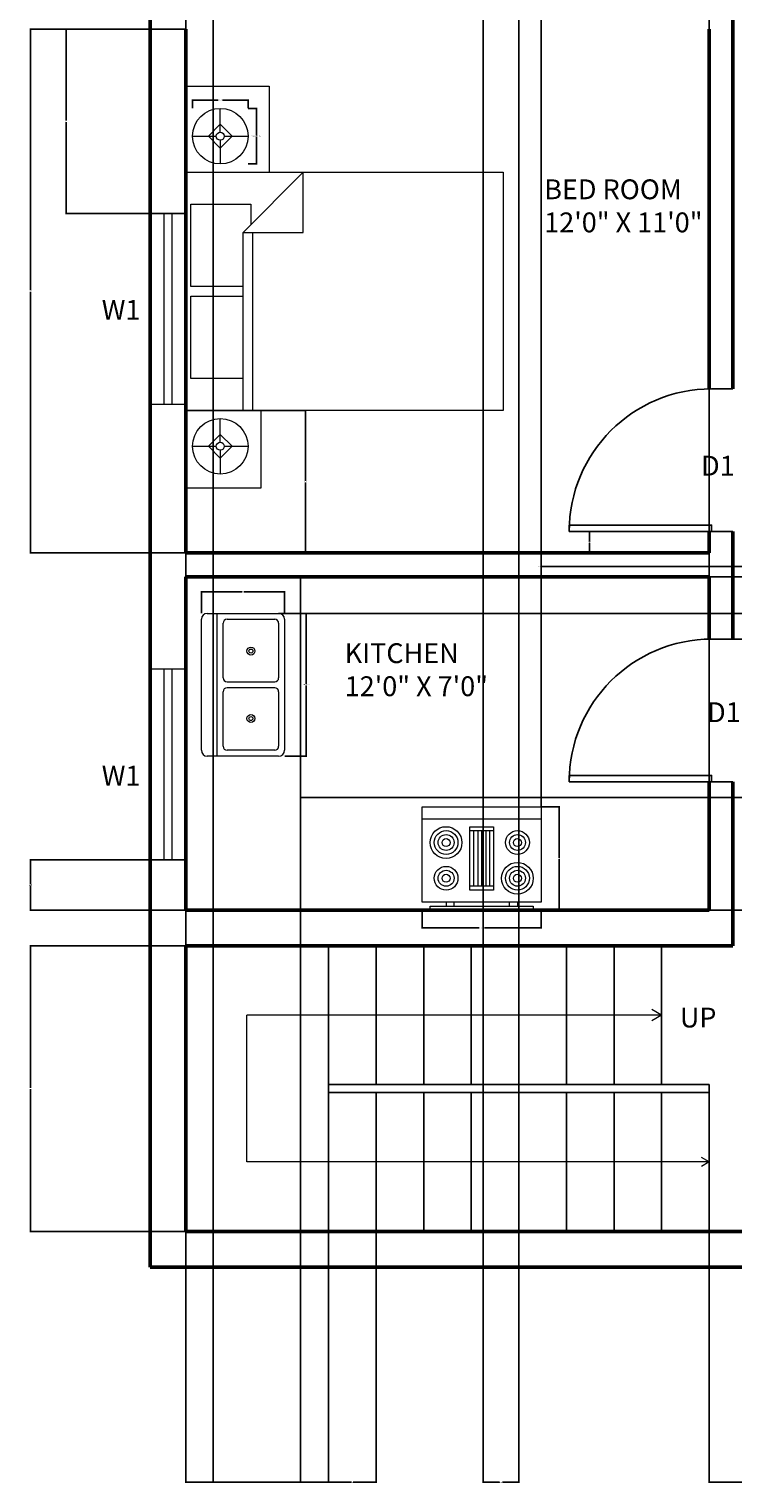
# Model space of a CAD drawing. Units: inches. Extents: x 437 to 811, y 2074 to 2699.
# Tile 1 of 4: x 437 to 615, y 2074 to 2441. Entities that reach past the tile are written whole.
import ezdxf

# ---------------------------------------------------------------- set-up
doc = ezdxf.new("R2010")
doc.units = ezdxf.units.IN
for name, color, linetype, lineweight in [('A-ANNO-DIMS', 2, 'Continuous', 18), ('A-ANNO-SYMB', 3, 'Continuous', 18), ('A-ANNO-TEXT', 7, 'Continuous', 18), ('A-AREA-IDEN', 7, 'Continuous', 25), ('A-DOOR', 4, 'Continuous', 25), ('A-EQPM', 8, 'Continuous', 18), ('A-FLOR-CASE', 9, 'Continuous', 25), ('A-FLOR-FIXT', 9, 'Continuous', 18), ('A-FLOR-STRS', 7, 'Continuous', 25), ('A-FURN', 8, 'Continuous', 18), ('A-GLAZ', 4, 'Continuous', 18), ('A-WALL', 7, 'Continuous', 50)]:
    doc.layers.add(name, color=color, linetype=linetype, lineweight=lineweight)
doc.styles.get("Standard").update_dxf_attribs({"font": 'arial.ttf'})
doc.dimstyles.get("Standard").update_dxf_attribs({"dimtxt": 0.18, "dimasz": 0.18, "dimexe": 0.18, "dimexo": 0.0625, "dimgap": 0.09, "dimtad": 0, "dimtih": 1, "dimtoh": 1, "dimdec": 4, "dimzin": 0, "dimdsep": 46, "dimtxsty": 'Standard', "dimcen": 0.09, "dimadec": 0, "dimazin": 0, "dimtfac": 1, "dimtdec": 4, "dimtofl": 0, "dimtmove": 0, "dimatfit": 3, "dimfxl": 1, "dimtolj": 1, "dimtzin": 0, "dimarcsym": 0})

# ---------------------------------------------------------------- blocks, each defined once
blk = doc.blocks.new('Range-Oven - 30 in top')
for p, q in [((0, -3), (30, -3)), ((12, -6), (18, -6)), ((13, -20), (13, -6)), ((14, -6), (14, -20)), ((15, -20), (15, -6)), ((16, -6), (16, -20)), ((17, -20), (17, -6)), ((18, -20), (12, -20)), ((6, -24), (6, -25)), ((8, -25), (8, -24)), ((22, -25), (22, -24)), ((24, -24), (24, -25))]:
    blk.add_line(p, q)
for points in [[(0, -24), (0, 0), (30, 0), (30, -24)], [(12, -21), (12, -5), (18, -5), (18, -21)], [(2, -26), (2, -25), (28, -25), (28, -26)]]:
    blk.add_lwpolyline(points, close=True)
for centre, radius in [((6, -9), 4), ((6, -9), 3), ((6, -9), 2), ((24, -9), 3), ((24, -9), 2), ((6, -9), 1), ((24, -9), 1), ((24, -18), 4), ((6, -18), 3), ((6, -18), 2), ((6, -18), 1), ((24, -18), 3), ((24, -18), 2), ((24, -18), 1)]:
    blk.add_circle(centre, radius)
blk = doc.blocks.new('Sink-double - 36 in top')
for p, q in [((-18, -4), (18, -4)), ((-0.75, -18.5), (-0.75, -6.5)), ((0.75, -6.5), (0.75, -18.5))]:
    blk.add_line(p, q)
for points in [[(-16.5, 0), (16.5, 0)], [(-18, -19.5), (-18, -1.5)], [(18, -1.5), (18, -19.5)], [(-16.5, -18.5), (-16.5, -6.5)], [(-15.5, -5.5), (-1.75, -5.5)], [(1.75, -5.5), (15.5, -5.5)], [(16.5, -6.5), (16.5, -18.5)], [(16.5, -21), (-16.5, -21)], [(-1.75, -19.5), (-15.5, -19.5)], [(15.5, -19.5), (1.75, -19.5)]]:
    blk.add_lwpolyline(points)
for centre, radius in [((-8.5, -12.5), 1), ((-8.5, -12.5), 0.5), ((8.5, -12.5), 1), ((8.5, -12.5), 0.5)]:
    blk.add_circle(centre, radius)
for centre, radius, start, end in [((-16.5, -1.5), 1.5, 90, 180), ((16.5, -1.5), 1.5, 0, 90), ((-15.5, -6.5), 1, 90, 180), ((-1.75, -6.5), 1, 0, 90), ((1.75, -6.5), 1, 90, 180), ((15.5, -6.5), 1, 0, 90), ((-16.5, -19.5), 1.5, 180, 270), ((-15.5, -18.5), 1, 180, 270), ((-1.75, -18.5), 1, 270, 0), ((1.75, -18.5), 1, 180, 270), ((15.5, -18.5), 1, 270, 0), ((16.5, -19.5), 1.5, 270, 0)]:
    blk.add_arc(centre, radius, start, end)
blk = doc.blocks.new('Bed - Queen')
for p, q in [((0, -80.00003), (0, 0)), ((0, 0), (59.99999, 0)), ((59.99999, 0), (59.99999, -80.00003)), ((7.99999, -1.2), (28.79998, -1.2)), ((7.99999, -14.4), (7.99999, -1.2)), ((28.79998, -1.2), (28.79998, -14.4)), ((31.19999, -1.2), (51.99999, -1.2)), ((31.19999, -14.4), (31.19999, -1.2)), ((51.99999, -1.2), (51.99999, -16.4)), ((0, -14.4), (44.8, -14.4)), ((59.99999, -29.6), (44.8, -14.4)), ((44.8, -14.4), (44.8, -29.6)), ((44.8, -16.8), (0, -16.8)), ((51.99999, -16.4), (46.79936, -16.4)), ((44.8, -29.6), (59.99999, -29.6)), ((59.99999, -80.00003), (0, -80.00003))]:
    blk.add_line(p, q)
blk = doc.blocks.new('Lamp - Table')
for p, q in [((0, 7), (0, 1)), ((-1, 0), (-7, 0)), ((0, 3), (-3, 0)), ((-3, 0), (0, -3)), ((3, 0), (0, 3)), ((0, -3), (3, 0)), ((1, 0), (7, 0)), ((0, -1), (0, -7))]:
    blk.add_line(p, q)
for radius in [7, 1]:
    blk.add_circle((0, 0), radius)
blk = doc.blocks.new('*U10')
for p, q in [((0, 0), (0, -6)), ((40, 0), (40, -6))]:
    blk.add_line(p, q)
blk.add_lwpolyline([(0, 0), (0, 40), (1.75, 40), (1.75, 0)], close=True)
blk.add_arc((0, 0), 40, 0, 90)
blk = doc.blocks.new('WIN-W1-48IN')
for p, q in [((0, 5.5), (48, 5.5)), ((0, 3.5), (48, 3.5))]:
    blk.add_line(p, q)
blk.add_lwpolyline([(0, 0), (48, 0), (48, 9), (0, 9)], close=True)
blk = doc.blocks.new('NIGHTSTAND-SMALL')
for p, q in [((0, 19.48), (0, 0)), ((19, 0), (19, 19.48)), ((0, 0), (19, 0))]:
    blk.add_line(p, q)
blk = doc.blocks.new('NIGHTSTAND-LARGE')
for p, q in [((0, 0), (0, 21.74)), ((0, 21.74), (21.02, 21.74)), ((21.02, 21.74), (21.02, 0))]:
    blk.add_line(p, q)
blk = doc.blocks.new('*D16')
at = {"layer": 'A-ANNO-DIMS', "color": 0, "lineweight": -2, "transparency": 16777216}
for p, q in [((492.74, 2420.81), (494.96, 2420.81)), ((494.78, 2420.63), (494.78, 2413.99)), ((494.78, 2406.99), (494.78, 2413.62)), ((492.74, 2406.81), (494.96, 2406.81))]:
    blk.add_line(p, q, dxfattribs=at)
at = {"layer": 'A-ANNO-DIMS', "color": 0, "transparency": 16777216}
for points in [[(494.75, 2420.63), (494.81, 2420.63), (494.78, 2420.81)], [(494.75, 2406.99), (494.81, 2406.99), (494.78, 2406.81)]]:
    blk.add_solid(points, dxfattribs=at)
at = {"layer": 'Defpoints', "color": 0, "transparency": 16777216}
for p in [(492.68, 2420.81), (494.78, 2420.81), (492.68, 2406.81)]:
    blk.add_point(p, dxfattribs=at)
at = {"layer": 'A-ANNO-DIMS', "color": 0, "transparency": 16777216, "insert": (494.78, 2413.81), "char_height": 0.18, "attachment_point": 5}
blk.add_mtext('\\A1;TABLE LAMP 14 TYP.', dxfattribs=at)
blk = doc.blocks.new('*D17')
at = {"layer": 'A-ANNO-DIMS', "color": 0, "lineweight": -2, "transparency": 16777216}
for p, q in [((478.68, 2420.87), (478.68, 2423.09)), ((478.86, 2422.91), (485.16, 2422.91)), ((492.5, 2422.91), (486.2, 2422.91)), ((492.68, 2420.87), (492.68, 2423.09))]:
    blk.add_line(p, q, dxfattribs=at)
at = {"layer": 'A-ANNO-DIMS', "color": 0, "transparency": 16777216}
for points in [[(478.86, 2422.94), (478.86, 2422.88), (478.68, 2422.91)], [(492.5, 2422.94), (492.5, 2422.88), (492.68, 2422.91)]]:
    blk.add_solid(points, dxfattribs=at)
at = {"layer": 'Defpoints', "color": 0, "transparency": 16777216}
for p in [(478.68, 2422.91), (478.68, 2420.81), (492.68, 2420.81)]:
    blk.add_point(p, dxfattribs=at)
at = {"layer": 'A-ANNO-DIMS', "color": 0, "transparency": 16777216, "insert": (485.68, 2422.91), "char_height": 0.18, "attachment_point": 5}
blk.add_mtext('\\A1;14 TYP.', dxfattribs=at)
blk = doc.blocks.new('*D38')
at = {"layer": 'A-ANNO-DIMS', "color": 0, "lineweight": -2, "transparency": 16777216}
for p, q in [((536.64, 2218.74), (536.64, 2214.12)), ((566.64, 2218.74), (566.64, 2214.12)), ((536.82, 2214.3), (550.94, 2214.3)), ((566.46, 2214.3), (552.33, 2214.3))]:
    blk.add_line(p, q, dxfattribs=at)
at = {"layer": 'A-ANNO-DIMS', "color": 0, "transparency": 16777216}
for points in [[(536.82, 2214.33), (536.82, 2214.27), (536.64, 2214.3)], [(566.46, 2214.33), (566.46, 2214.27), (566.64, 2214.3)]]:
    blk.add_solid(points, dxfattribs=at)
at = {"layer": 'Defpoints', "color": 0, "transparency": 16777216}
for p in [(536.64, 2218.8), (566.64, 2218.8), (566.64, 2214.3)]:
    blk.add_point(p, dxfattribs=at)
at = {"layer": 'A-ANNO-DIMS', "color": 0, "transparency": 16777216, "insert": (551.64, 2214.3), "char_height": 0.18, "attachment_point": 5}
blk.add_mtext('\\A1;RANGE 30', dxfattribs=at)
blk = doc.blocks.new('*D39')
at = {"layer": 'A-ANNO-DIMS', "color": 0, "lineweight": -2, "transparency": 16777216}
for p, q in [((566.7, 2244.8), (571.32, 2244.8)), ((571.14, 2244.62), (571.14, 2231.98)), ((571.14, 2218.98), (571.14, 2231.62)), ((566.7, 2218.8), (571.32, 2218.8))]:
    blk.add_line(p, q, dxfattribs=at)
at = {"layer": 'A-ANNO-DIMS', "color": 0, "transparency": 16777216}
for points in [[(571.11, 2244.62), (571.17, 2244.62), (571.14, 2244.8)], [(571.11, 2218.98), (571.17, 2218.98), (571.14, 2218.8)]]:
    blk.add_solid(points, dxfattribs=at)
at = {"layer": 'Defpoints', "color": 0, "transparency": 16777216}
for p in [(566.64, 2244.8), (571.14, 2244.8), (566.64, 2218.8)]:
    blk.add_point(p, dxfattribs=at)
at = {"layer": 'A-ANNO-DIMS', "color": 0, "transparency": 16777216, "insert": (571.14, 2231.8), "char_height": 0.18, "attachment_point": 5}
blk.add_mtext('\\A1;26', dxfattribs=at)
blk = doc.blocks.new('*D40')
at = {"layer": 'A-ANNO-DIMS', "color": 0, "lineweight": -2, "transparency": 16777216}
for p, q in [((501.96, 2293.56), (507.48, 2293.56)), ((507.3, 2293.38), (507.3, 2275.74)), ((507.3, 2257.74), (507.3, 2275.37)), ((501.96, 2257.56), (507.48, 2257.56))]:
    blk.add_line(p, q, dxfattribs=at)
at = {"layer": 'A-ANNO-DIMS', "color": 0, "transparency": 16777216}
for points in [[(507.27, 2293.38), (507.33, 2293.38), (507.3, 2293.56)], [(507.27, 2257.74), (507.33, 2257.74), (507.3, 2257.56)]]:
    blk.add_solid(points, dxfattribs=at)
at = {"layer": 'Defpoints', "color": 0, "transparency": 16777216}
for p in [(501.9, 2293.56), (507.3, 2293.56), (501.9, 2257.56)]:
    blk.add_point(p, dxfattribs=at)
at = {"layer": 'A-ANNO-DIMS', "color": 0, "transparency": 16777216, "insert": (507.3, 2275.56), "char_height": 0.18, "attachment_point": 5}
blk.add_mtext('\\A1;DOUBLE SINK 36', dxfattribs=at)
blk = doc.blocks.new('*D41')
at = {"layer": 'A-ANNO-DIMS', "color": 0, "lineweight": -2, "transparency": 16777216}
for p, q in [((480.9, 2293.62), (480.9, 2299.14)), ((481.08, 2298.96), (491.2, 2298.96)), ((501.72, 2298.96), (491.6, 2298.96)), ((501.9, 2293.62), (501.9, 2299.14))]:
    blk.add_line(p, q, dxfattribs=at)
at = {"layer": 'A-ANNO-DIMS', "color": 0, "transparency": 16777216}
for points in [[(481.08, 2298.99), (481.08, 2298.93), (480.9, 2298.96)], [(501.72, 2298.99), (501.72, 2298.93), (501.9, 2298.96)]]:
    blk.add_solid(points, dxfattribs=at)
at = {"layer": 'Defpoints', "color": 0, "transparency": 16777216}
for p in [(480.9, 2298.96), (480.9, 2293.56), (501.9, 2293.56)]:
    blk.add_point(p, dxfattribs=at)
at = {"layer": 'A-ANNO-DIMS', "color": 0, "transparency": 16777216, "insert": (491.4, 2298.96), "char_height": 0.18, "attachment_point": 5}
blk.add_mtext('\\A1;21', dxfattribs=at)
blk = doc.blocks.new('*D44')
at = {"layer": 'A-ANNO-DIMS', "color": 0, "lineweight": -2, "transparency": 16777216}
for p, q in [((609, 2137.74), (609, 2074.42)), ((645.69, 2104.74), (645.69, 2074.42)), ((609.18, 2074.6), (626.95, 2074.6)), ((645.51, 2074.6), (627.74, 2074.6))]:
    blk.add_line(p, q, dxfattribs=at)
at = {"layer": 'A-ANNO-DIMS', "color": 0, "transparency": 16777216}
for points in [[(609.18, 2074.63), (609.18, 2074.57), (609, 2074.6)], [(645.51, 2074.63), (645.51, 2074.57), (645.69, 2074.6)]]:
    blk.add_solid(points, dxfattribs=at)
at = {"layer": 'Defpoints', "color": 0, "transparency": 16777216}
for p in [(609, 2137.8), (645.69, 2104.8), (645.69, 2074.6)]:
    blk.add_point(p, dxfattribs=at)
at = {"layer": 'A-ANNO-DIMS', "color": 0, "transparency": 16777216, "insert": (627.35, 2074.6), "char_height": 0.18, "attachment_point": 5}
blk.add_mtext('\\A1;36.69', dxfattribs=at)
blk = doc.blocks.new('*D51')
at = {"layer": 'A-ANNO-DIMS', "color": 0, "lineweight": -2, "transparency": 16777216}
for p, q in [((476.94, 2231.48), (437.62, 2231.48)), ((437.8, 2231.3), (437.8, 2225.32)), ((437.8, 2218.98), (437.8, 2224.96)), ((476.94, 2218.8), (437.62, 2218.8))]:
    blk.add_line(p, q, dxfattribs=at)
at = {"layer": 'A-ANNO-DIMS', "color": 0, "transparency": 16777216}
for points in [[(437.77, 2231.3), (437.83, 2231.3), (437.8, 2231.48)], [(437.77, 2218.98), (437.83, 2218.98), (437.8, 2218.8)]]:
    blk.add_solid(points, dxfattribs=at)
at = {"layer": 'Defpoints', "color": 0, "transparency": 16777216}
for p in [(437.8, 2231.48), (477, 2231.48), (477, 2218.8)]:
    blk.add_point(p, dxfattribs=at)
at = {"layer": 'A-ANNO-DIMS', "color": 0, "transparency": 16777216, "insert": (437.8, 2225.14), "char_height": 0.18, "attachment_point": 5}
blk.add_mtext('\\A1;12.684', dxfattribs=at)
blk = doc.blocks.new('*D52')
at = {"layer": 'A-ANNO-DIMS', "color": 0, "lineweight": -2, "transparency": 16777216}
for p, q in [((476.94, 2440.8), (446.62, 2440.8)), ((446.8, 2440.62), (446.8, 2417.73)), ((446.8, 2394.48), (446.8, 2417.37)), ((476.94, 2394.3), (446.62, 2394.3))]:
    blk.add_line(p, q, dxfattribs=at)
at = {"layer": 'A-ANNO-DIMS', "color": 0, "transparency": 16777216}
for points in [[(446.77, 2440.62), (446.83, 2440.62), (446.8, 2440.8)], [(446.77, 2394.48), (446.83, 2394.48), (446.8, 2394.3)]]:
    blk.add_solid(points, dxfattribs=at)
at = {"layer": 'Defpoints', "color": 0, "transparency": 16777216}
for p in [(446.8, 2440.8), (477, 2440.8), (477, 2394.3)]:
    blk.add_point(p, dxfattribs=at)
at = {"layer": 'A-ANNO-DIMS', "color": 0, "transparency": 16777216, "insert": (446.8, 2417.55), "char_height": 0.18, "attachment_point": 5}
blk.add_mtext('\\A1;46.5', dxfattribs=at)
blk = doc.blocks.new('*D53')
at = {"layer": 'A-ANNO-DIMS', "color": 0, "lineweight": -2, "transparency": 16777216}
for p, q in [((476.94, 2440.8), (437.62, 2440.8)), ((437.8, 2440.62), (437.8, 2374.98)), ((437.8, 2308.98), (437.8, 2374.62)), ((476.94, 2308.8), (437.62, 2308.8))]:
    blk.add_line(p, q, dxfattribs=at)
at = {"layer": 'A-ANNO-DIMS', "color": 0, "transparency": 16777216}
for points in [[(437.77, 2440.62), (437.83, 2440.62), (437.8, 2440.8)], [(437.77, 2308.98), (437.83, 2308.98), (437.8, 2308.8)]]:
    blk.add_solid(points, dxfattribs=at)
at = {"layer": 'Defpoints', "color": 0, "transparency": 16777216}
for p in [(437.8, 2440.8), (477, 2440.8), (477, 2308.8)]:
    blk.add_point(p, dxfattribs=at)
at = {"layer": 'A-ANNO-DIMS', "color": 0, "transparency": 16777216, "insert": (437.8, 2374.8), "char_height": 0.18, "attachment_point": 5}
blk.add_mtext('\\A1;132', dxfattribs=at)
blk = doc.blocks.new('*D61')
at = {"layer": 'A-ANNO-DIMS', "color": 0, "lineweight": -2, "transparency": 16777216}
for p, q in [((476.94, 2209.8), (437.62, 2209.8)), ((437.8, 2209.62), (437.8, 2173.98)), ((437.8, 2137.98), (437.8, 2173.62)), ((476.94, 2137.8), (437.62, 2137.8))]:
    blk.add_line(p, q, dxfattribs=at)
at = {"layer": 'A-ANNO-DIMS', "color": 0, "transparency": 16777216}
for points in [[(437.77, 2209.62), (437.83, 2209.62), (437.8, 2209.8)], [(437.77, 2137.98), (437.83, 2137.98), (437.8, 2137.8)]]:
    blk.add_solid(points, dxfattribs=at)
at = {"layer": 'Defpoints', "color": 0, "transparency": 16777216}
for p in [(437.8, 2209.8), (477, 2209.8), (477, 2137.8)]:
    blk.add_point(p, dxfattribs=at)
at = {"layer": 'A-ANNO-DIMS', "color": 0, "transparency": 16777216, "insert": (437.8, 2173.8), "char_height": 0.18, "attachment_point": 5}
blk.add_mtext('\\A1;72', dxfattribs=at)
blk = doc.blocks.new('*D62')
at = {"layer": 'A-ANNO-DIMS', "color": 0, "lineweight": -2, "transparency": 16777216}
for p, q in [((477, 2137.74), (477, 2074.42)), ((513, 2137.74), (513, 2074.42)), ((477.18, 2074.6), (494.79, 2074.6)), ((512.82, 2074.6), (495.22, 2074.6))]:
    blk.add_line(p, q, dxfattribs=at)
at = {"layer": 'A-ANNO-DIMS', "color": 0, "transparency": 16777216}
for points in [[(477.18, 2074.63), (477.18, 2074.57), (477, 2074.6)], [(512.82, 2074.63), (512.82, 2074.57), (513, 2074.6)]]:
    blk.add_solid(points, dxfattribs=at)
at = {"layer": 'Defpoints', "color": 0, "transparency": 16777216}
for p in [(477, 2137.8), (513, 2137.8), (513, 2074.6)]:
    blk.add_point(p, dxfattribs=at)
at = {"layer": 'A-ANNO-DIMS', "color": 0, "transparency": 16777216, "insert": (495, 2074.6), "char_height": 0.18, "attachment_point": 5}
blk.add_mtext('\\A1;36', dxfattribs=at)
blk = doc.blocks.new('*D63')
at = {"layer": 'A-ANNO-DIMS', "color": 0, "lineweight": -2, "transparency": 16777216}
for p, q in [((513, 2137.74), (513, 2074.42)), ((525, 2137.74), (525, 2074.42)), ((513.18, 2074.6), (518.8, 2074.6)), ((524.82, 2074.6), (519.21, 2074.6))]:
    blk.add_line(p, q, dxfattribs=at)
at = {"layer": 'A-ANNO-DIMS', "color": 0, "transparency": 16777216}
for points in [[(513.18, 2074.63), (513.18, 2074.57), (513, 2074.6)], [(524.82, 2074.63), (524.82, 2074.57), (525, 2074.6)]]:
    blk.add_solid(points, dxfattribs=at)
at = {"layer": 'Defpoints', "color": 0, "transparency": 16777216}
for p in [(513, 2137.8), (525, 2137.8), (525, 2074.6)]:
    blk.add_point(p, dxfattribs=at)
at = {"layer": 'A-ANNO-DIMS', "color": 0, "transparency": 16777216, "insert": (519, 2074.6), "char_height": 0.18, "attachment_point": 5}
blk.add_mtext('\\A1;12', dxfattribs=at)
blk = doc.blocks.new('*D65')
at = {"layer": 'A-ANNO-DIMS', "color": 0, "lineweight": -2, "transparency": 16777216}
for p, q in [((609.07, 2302.8), (810.38, 2302.8)), ((810.2, 2302.62), (810.2, 2295.11)), ((810.2, 2287.23), (810.2, 2294.74)), ((609.07, 2287.05), (810.38, 2287.05))]:
    blk.add_line(p, q, dxfattribs=at)
at = {"layer": 'A-ANNO-DIMS', "color": 0, "transparency": 16777216}
for points in [[(810.17, 2302.62), (810.23, 2302.62), (810.2, 2302.8)], [(810.17, 2287.23), (810.23, 2287.23), (810.2, 2287.05)]]:
    blk.add_solid(points, dxfattribs=at)
at = {"layer": 'Defpoints', "color": 0, "transparency": 16777216}
for p in [(609, 2302.8), (810.2, 2302.8), (609, 2287.05)]:
    blk.add_point(p, dxfattribs=at)
at = {"layer": 'A-ANNO-DIMS', "color": 0, "transparency": 16777216, "insert": (810.2, 2294.93), "char_height": 0.18, "attachment_point": 5}
blk.add_mtext('\\A1;15.747', dxfattribs=at)
blk = doc.blocks.new('*D66')
at = {"layer": 'A-ANNO-DIMS', "color": 0, "lineweight": -2, "transparency": 16777216}
for p, q in [((477, 2302.86), (477, 2690.18)), ((477.18, 2690), (542.73, 2690)), ((608.82, 2690), (543.28, 2690)), ((609, 2302.86), (609, 2690.18))]:
    blk.add_line(p, q, dxfattribs=at)
at = {"layer": 'A-ANNO-DIMS', "color": 0, "transparency": 16777216}
for points in [[(477.18, 2690.03), (477.18, 2689.97), (477, 2690)], [(608.82, 2690.03), (608.82, 2689.97), (609, 2690)]]:
    blk.add_solid(points, dxfattribs=at)
at = {"layer": 'Defpoints', "color": 0, "transparency": 16777216}
for p in [(609, 2690), (477, 2302.8), (609, 2302.8)]:
    blk.add_point(p, dxfattribs=at)
at = {"layer": 'A-ANNO-DIMS', "color": 0, "transparency": 16777216, "insert": (543, 2690), "char_height": 0.18, "attachment_point": 5}
blk.add_mtext('\\A1;132', dxfattribs=at)
blk = doc.blocks.new('*D67')
at = {"layer": 'A-ANNO-DIMS', "color": 0, "lineweight": -2, "transparency": 16777216}
for p, q in [((505.92, 2247.12), (505.92, 2074.42)), ((477, 2218.74), (477, 2074.42)), ((477.18, 2074.6), (491, 2074.6)), ((505.74, 2074.6), (491.93, 2074.6))]:
    blk.add_line(p, q, dxfattribs=at)
at = {"layer": 'A-ANNO-DIMS', "color": 0, "transparency": 16777216}
for points in [[(477.18, 2074.63), (477.18, 2074.57), (477, 2074.6)], [(505.74, 2074.63), (505.74, 2074.57), (505.92, 2074.6)]]:
    blk.add_solid(points, dxfattribs=at)
at = {"layer": 'Defpoints', "color": 0, "transparency": 16777216}
for p in [(505.92, 2247.18), (477, 2218.8), (505.92, 2074.6)]:
    blk.add_point(p, dxfattribs=at)
at = {"layer": 'A-ANNO-DIMS', "color": 0, "transparency": 16777216, "insert": (491.46, 2074.6), "char_height": 0.18, "attachment_point": 5}
blk.add_mtext('\\A1;28.916', dxfattribs=at)
blk = doc.blocks.new('*D68')
at = {"layer": 'A-ANNO-DIMS', "color": 0, "lineweight": -2, "transparency": 16777216}
for p, q in [((609.07, 2247.18), (810.38, 2247.18)), ((810.2, 2247), (810.2, 2233.17)), ((810.2, 2218.98), (810.2, 2232.81)), ((609.07, 2218.8), (810.38, 2218.8))]:
    blk.add_line(p, q, dxfattribs=at)
at = {"layer": 'A-ANNO-DIMS', "color": 0, "transparency": 16777216}
for points in [[(810.17, 2247), (810.23, 2247), (810.2, 2247.18)], [(810.17, 2218.98), (810.23, 2218.98), (810.2, 2218.8)]]:
    blk.add_solid(points, dxfattribs=at)
at = {"layer": 'Defpoints', "color": 0, "transparency": 16777216}
for p in [(609, 2247.18), (810.2, 2247.18), (609, 2218.8)]:
    blk.add_point(p, dxfattribs=at)
at = {"layer": 'A-ANNO-DIMS', "color": 0, "transparency": 16777216, "insert": (810.2, 2232.99), "char_height": 0.18, "attachment_point": 5}
blk.add_mtext('\\A1;28.384', dxfattribs=at)
blk = doc.blocks.new('*D69')
at = {"layer": 'A-ANNO-DIMS', "color": 0, "lineweight": -2, "transparency": 16777216}
for p, q in [((566.64, 2244.86), (566.64, 2690.18)), ((566.82, 2690), (587.42, 2690)), ((608.82, 2690), (588.22, 2690)), ((609, 2247.25), (609, 2690.18))]:
    blk.add_line(p, q, dxfattribs=at)
at = {"layer": 'A-ANNO-DIMS', "color": 0, "transparency": 16777216}
for points in [[(566.82, 2690.03), (566.82, 2689.97), (566.64, 2690)], [(608.82, 2690.03), (608.82, 2689.97), (609, 2690)]]:
    blk.add_solid(points, dxfattribs=at)
at = {"layer": 'Defpoints', "color": 0, "transparency": 16777216}
for p in [(609, 2690), (609, 2247.18), (566.64, 2244.8)]:
    blk.add_point(p, dxfattribs=at)
at = {"layer": 'A-ANNO-DIMS', "color": 0, "transparency": 16777216, "insert": (587.82, 2690), "char_height": 0.18, "attachment_point": 5}
blk.add_mtext('\\A1;42.37', dxfattribs=at)
blk = doc.blocks.new('*D70')
at = {"layer": 'A-ANNO-DIMS', "color": 0, "lineweight": -2, "transparency": 16777216}
for p, q in [((505.98, 2302.8), (810.38, 2302.8)), ((810.2, 2302.62), (810.2, 2298.36)), ((810.2, 2293.74), (810.2, 2298)), ((500.46, 2293.56), (810.38, 2293.56))]:
    blk.add_line(p, q, dxfattribs=at)
at = {"layer": 'A-ANNO-DIMS', "color": 0, "transparency": 16777216}
for points in [[(810.17, 2302.62), (810.23, 2302.62), (810.2, 2302.8)], [(810.17, 2293.74), (810.23, 2293.74), (810.2, 2293.56)]]:
    blk.add_solid(points, dxfattribs=at)
at = {"layer": 'Defpoints', "color": 0, "transparency": 16777216}
for p in [(505.92, 2302.8), (810.2, 2302.8), (500.4, 2293.56)]:
    blk.add_point(p, dxfattribs=at)
at = {"layer": 'A-ANNO-DIMS', "color": 0, "transparency": 16777216, "insert": (810.2, 2298.18), "char_height": 0.18, "attachment_point": 5}
blk.add_mtext('\\A1;9.244', dxfattribs=at)
blk = doc.blocks.new('*D71')
at = {"layer": 'A-ANNO-DIMS', "color": 0, "lineweight": -2, "transparency": 16777216}
for p, q in [((477, 2446.74), (477, 2074.42)), ((483.87, 2446.74), (483.87, 2074.42)), ((477.18, 2074.6), (480.04, 2074.6)), ((483.69, 2074.6), (480.83, 2074.6))]:
    blk.add_line(p, q, dxfattribs=at)
at = {"layer": 'A-ANNO-DIMS', "color": 0, "transparency": 16777216}
for points in [[(477.18, 2074.63), (477.18, 2074.57), (477, 2074.6)], [(483.69, 2074.63), (483.69, 2074.57), (483.87, 2074.6)]]:
    blk.add_solid(points, dxfattribs=at)
at = {"layer": 'Defpoints', "color": 0, "transparency": 16777216}
for p in [(477, 2446.8), (483.87, 2446.8), (483.87, 2074.6)]:
    blk.add_point(p, dxfattribs=at)
at = {"layer": 'A-ANNO-DIMS', "color": 0, "transparency": 16777216, "insert": (480.44, 2074.6), "char_height": 0.18, "attachment_point": 5}
blk.add_mtext('\\A1;6.864', dxfattribs=at)
blk = doc.blocks.new('*D73')
at = {"layer": 'A-ANNO-DIMS', "color": 0, "lineweight": -2, "transparency": 16777216}
for p, q in [((551.96, 2446.74), (551.96, 2074.42)), ((561, 2446.74), (561, 2074.42)), ((552.14, 2074.6), (556.09, 2074.6)), ((560.82, 2074.6), (556.88, 2074.6))]:
    blk.add_line(p, q, dxfattribs=at)
at = {"layer": 'A-ANNO-DIMS', "color": 0, "transparency": 16777216}
for points in [[(552.14, 2074.63), (552.14, 2074.57), (551.96, 2074.6)], [(560.82, 2074.63), (560.82, 2074.57), (561, 2074.6)]]:
    blk.add_solid(points, dxfattribs=at)
at = {"layer": 'Defpoints', "color": 0, "transparency": 16777216}
for p in [(551.96, 2446.8), (561, 2446.8), (561, 2074.6)]:
    blk.add_point(p, dxfattribs=at)
at = {"layer": 'A-ANNO-DIMS', "color": 0, "transparency": 16777216, "insert": (556.48, 2074.6), "char_height": 0.18, "attachment_point": 5}
blk.add_mtext('\\A1;9.045', dxfattribs=at)
blk = doc.blocks.new('*D74')
at = {"layer": 'A-ANNO-DIMS', "color": 0, "lineweight": -2, "transparency": 16777216}
for p, q in [((608.94, 2314.22), (578.62, 2314.22)), ((578.8, 2314.04), (578.8, 2311.69)), ((608.94, 2308.8), (578.62, 2308.8)), ((578.8, 2308.98), (578.8, 2311.33))]:
    blk.add_line(p, q, dxfattribs=at)
at = {"layer": 'A-ANNO-DIMS', "color": 0, "transparency": 16777216}
for points in [[(578.77, 2314.04), (578.83, 2314.04), (578.8, 2314.22)], [(578.77, 2308.98), (578.83, 2308.98), (578.8, 2308.8)]]:
    blk.add_solid(points, dxfattribs=at)
at = {"layer": 'Defpoints', "color": 0, "transparency": 16777216}
for p in [(578.8, 2314.22), (609, 2314.22), (609, 2308.8)]:
    blk.add_point(p, dxfattribs=at)
at = {"layer": 'A-ANNO-DIMS', "color": 0, "transparency": 16777216, "insert": (578.8, 2311.51), "char_height": 0.18, "attachment_point": 5}
blk.add_mtext('\\A1;5.416', dxfattribs=at)
blk = doc.blocks.new('*D81')
at = {"layer": 'A-ANNO-DIMS', "color": 0, "lineweight": -2, "transparency": 16777216}
for p, q in [((477.07, 2344.71), (507.38, 2344.71)), ((507.2, 2344.53), (507.2, 2326.93)), ((507.2, 2308.98), (507.2, 2326.57)), ((477.07, 2308.8), (507.38, 2308.8))]:
    blk.add_line(p, q, dxfattribs=at)
at = {"layer": 'A-ANNO-DIMS', "color": 0, "transparency": 16777216}
for points in [[(507.17, 2344.53), (507.23, 2344.53), (507.2, 2344.71)], [(507.17, 2308.98), (507.23, 2308.98), (507.2, 2308.8)]]:
    blk.add_solid(points, dxfattribs=at)
at = {"layer": 'Defpoints', "color": 0, "transparency": 16777216}
for p in [(477, 2344.71), (477, 2308.8), (507.2, 2308.8)]:
    blk.add_point(p, dxfattribs=at)
at = {"layer": 'A-ANNO-DIMS', "color": 0, "transparency": 16777216, "insert": (507.2, 2326.75), "char_height": 0.18, "attachment_point": 5}
blk.add_mtext('\\A1;35.906', dxfattribs=at)
blk = doc.blocks.new('*D88')
at = {"layer": 'A-ANNO-DIMS', "color": 0, "lineweight": -2, "transparency": 16777216}
for p, q in [((568.95, 2305.38), (641.01, 2305.38)), ((762.3, 2305.38), (762.48, 2305.38)), ((762.39, 2305.29), (762.39, 2305.47))]:
    blk.add_line(p, q, dxfattribs=at)
at = {"layer": 'A-ANNO-DIMS', "color": 0, "transparency": 16777216}
blk.add_solid([(641.01, 2305.41), (641.01, 2305.35), (641.19, 2305.38)], dxfattribs=at)
at = {"layer": 'Defpoints', "color": 0, "transparency": 16777216}
for p in [(641.19, 2305.38), (762.39, 2305.38)]:
    blk.add_point(p, dxfattribs=at)
at = {"layer": 'A-ANNO-DIMS', "color": 0, "transparency": 16777216, "insert": (568.47, 2305.38), "char_height": 0.18, "attachment_point": 5}
blk.add_mtext('\\A1;R121.2', dxfattribs=at)
blk = doc.blocks.new('*D89')
at = {"layer": 'A-ANNO-DIMS', "color": 0, "lineweight": -2, "transparency": 16777216}
for p, q in [((566.64, 2305.38), (635.01, 2305.38)), ((749.35, 2305.38), (749.53, 2305.38)), ((749.44, 2305.29), (749.44, 2305.47))]:
    blk.add_line(p, q, dxfattribs=at)
at = {"layer": 'A-ANNO-DIMS', "color": 0, "transparency": 16777216}
blk.add_solid([(635.01, 2305.41), (635.01, 2305.35), (635.19, 2305.38)], dxfattribs=at)
at = {"layer": 'Defpoints', "color": 0, "transparency": 16777216}
for p in [(635.19, 2305.38), (749.44, 2305.38)]:
    blk.add_point(p, dxfattribs=at)
at = {"layer": 'A-ANNO-DIMS', "color": 0, "transparency": 16777216, "insert": (566.09, 2305.38), "char_height": 0.18, "attachment_point": 5}
blk.add_mtext('\\A1;R114.25', dxfattribs=at)

msp = doc.modelspace()

# ---------------------------------------------------------------- linework, layer by layer
at = {"layer": 'A-ANNO-SYMB'}
for p, q in [((597.0049, 2192.2995), (492.3677, 2192.2995)), ((492.3677, 2155.2995), (492.3677, 2192.2995)), ((597.0049, 2192.2995), (594.5087, 2193.7406)), ((597.0049, 2192.2995), (594.5087, 2190.8583)), ((609.0049, 2155.2995), (492.3677, 2155.2995)), ((609.0049, 2155.2995), (607.0775, 2156.4122)), ((609.0049, 2155.2995), (607.0775, 2154.1867))]:
    msp.add_line(p, q, dxfattribs=at)
at = {"layer": 'A-FLOR-CASE'}
for p, q in [((505.9211, 2302.7995), (505.9211, 2247.1838)), ((505.9211, 2247.1838), (609.0049, 2247.1838))]:
    msp.add_line(p, q, dxfattribs=at)
at = {"layer": 'A-FLOR-STRS'}
for p, q in [((477.0049, 2209.7995), (477.0049, 2137.7995)), ((513.0049, 2209.7995), (513.0049, 2137.7995)), ((525.0049, 2209.7995), (525.0049, 2174.7995)), ((537.0049, 2209.7995), (537.0049, 2174.7995)), ((549.0049, 2209.7995), (549.0049, 2174.7995)), ((561.0049, 2209.7995), (561.0049, 2174.7995)), ((573.0049, 2209.7995), (573.0049, 2174.7995)), ((585.0049, 2209.7995), (585.0049, 2174.7995)), ((597.0049, 2209.7995), (597.0049, 2174.7995)), ((609.0049, 2174.7995), (513.0049, 2174.7995)), ((609.0049, 2172.7995), (513.0049, 2172.7995)), ((525.0049, 2172.7995), (525.0049, 2137.7995)), ((537.0049, 2172.7995), (537.0049, 2137.7995)), ((549.0049, 2172.7995), (549.0049, 2137.7995)), ((561.0049, 2172.7995), (561.0049, 2137.7995)), ((573.0049, 2172.7995), (573.0049, 2137.7995)), ((585.0049, 2172.7995), (585.0049, 2137.7995)), ((597.0049, 2172.7995), (597.0049, 2137.7995)), ((609.0049, 2174.7995), (609.0049, 2172.7995)), ((609.0049, 2172.7995), (609.0049, 2137.7995))]:
    msp.add_line(p, q, dxfattribs=at)
at = {"layer": 'A-WALL'}
for p, q in [((468.0049, 2659.7995), (468.0049, 2128.7995)), ((615.0049, 2350.1394), (615.0049, 2446.7995)), ((477.0049, 2440.7995), (477.0049, 2308.7995)), ((609.0049, 2350.1342), (609.0049, 2440.7995)), ((609.0049, 2308.7995), (609.0049, 2314.2154)), ((615.0049, 2287.0573), (615.0049, 2314.2154)), ((477.0049, 2308.7995), (609.0049, 2308.7995)), ((477.0049, 2302.7995), (609.0049, 2302.7995)), ((477.0049, 2302.7995), (477.0049, 2218.7995)), ((609.0049, 2287.0521), (609.0049, 2302.7995)), ((609.0049, 2218.7995), (609.0049, 2251.1333)), ((615.0049, 2209.7995), (615.0049, 2251.1333)), ((477.0049, 2218.7995), (609.0049, 2218.7995)), ((477.0049, 2209.7995), (615.0049, 2209.7995)), ((477.0049, 2209.7995), (477.0049, 2137.7995)), ((477.0049, 2137.7995), (652.5955, 2137.7995)), ((468.0049, 2128.7995), (658.0738, 2128.7995))]:
    msp.add_line(p, q, dxfattribs=at)

# ---------------------------------------------------------------- block references
at = {"layer": 'A-DOOR', "xscale": 0.8981017077080947, "yscale": 0.8981017077080947, "zscale": 0.8981017077080947, "rotation": 90}
for p in [(609.6163, 2314.2154), (609.6163, 2251.1333)]:
    msp.add_blockref('*U10', p, dxfattribs=at)
at = {"layer": 'A-EQPM'}
msp.add_blockref('Range-Oven - 30 in top', (536.639, 2244.7994), dxfattribs=at)
at = {"layer": 'A-FLOR-FIXT', "rotation": 90}
msp.add_blockref('Sink-double - 36 in top', (480.9016, 2275.5551), dxfattribs=at)
at = {"layer": 'A-FURN'}
for name, p in [('NIGHTSTAND-LARGE', (477.005, 2404.706)), ('NIGHTSTAND-SMALL', (477.005, 2325.224))]:
    msp.add_blockref(name, p, dxfattribs=at)
at = {"layer": 'A-FURN', "rotation": 90}
for name, p in [('Lamp - Table', (485.6767, 2413.8051)), ('Bed - Queen', (477.0049, 2344.7056)), ('Lamp - Table', (485.6767, 2335.6608))]:
    msp.add_blockref(name, p, dxfattribs=at)
at = {"layer": 'A-GLAZ'}
for p, rotation in [((477.0053, 2346.2997), 89.99999999999928), ((477.0053, 2231.484), 89.99999999999945)]:
    msp.add_blockref('WIN-W1-48IN', p, dxfattribs=dict(at, rotation=rotation))

# ---------------------------------------------------------------- texts
at = {"layer": 'A-ANNO-TEXT', "char_height": 5, "width": 52.048983, "attachment_point": 1}
for s, insert in [('W1', (455.7597, 2372.5533)), ('D1', (606.9684, 2333.2659)), ('D1', (608.4809, 2271.1388)), ('W1', (455.7597, 2255.1569)), ('UP', (601.6095, 2194.1931))]:
    msp.add_mtext(s, dxfattribs=dict(at, insert=insert))
at = {"layer": 'A-AREA-IDEN', "char_height": 5, "width": 52.048983, "attachment_point": 1}
for s, insert in [('BED ROOM\\P12\'0" X 11\'0"', (567.3922, 2402.9191)), ('KITCHEN\\P12\'0" X 7\'0"', (517.0609, 2286.0206))]:
    msp.add_mtext(s, dxfattribs=dict(at, insert=insert))

# ---------------------------------------------------------------- dimensions: what is measured, and where the dimension line sits
at = {"layer": 'A-ANNO-DIMS'}
for base, p1, p2, override, picture, middle in [((609.0049, 2689.9995), (477.0049, 2302.7995), (609.0049, 2302.7995), {"dimdec": 0, "dimlfac": 1, "dimrnd": 0, "dimzin": 0, "dimdsep": 46, "dimlunit": 2}, '*D66', (543.0049, 2689.9995)), ((609.0049, 2689.9995), (566.639, 2244.7994), (609.0049, 2247.1838), {"dimdec": 2, "dimlfac": 1, "dimrnd": 0, "dimzin": 0, "dimdsep": 46, "dimlunit": 2}, '*D69', (587.8219, 2689.9995)), ((483.8691, 2074.5995), (477.0049, 2446.7995), (483.8691, 2446.7995), {"dimdec": 3, "dimlfac": 1, "dimrnd": 0, "dimzin": 0, "dimdsep": 46, "dimlunit": 2}, '*D71', (480.437, 2074.5995)), ((561.0049, 2074.5995), (551.9595, 2446.7995), (561.0049, 2446.7995), {"dimdec": 3, "dimlfac": 1, "dimrnd": 0, "dimzin": 0, "dimdsep": 46, "dimlunit": 2}, '*D73', (556.4822, 2074.5995)), ((505.9211, 2074.5995), (477.0049, 2218.7995), (505.9211, 2247.1838), {"dimdec": 3, "dimlfac": 1, "dimrnd": 0, "dimzin": 0, "dimdsep": 46, "dimlunit": 2}, '*D67', (491.463, 2074.5995)), ((513.0049, 2074.5995), (477.0049, 2137.7995), (513.0049, 2137.7995), {"dimdec": 0, "dimlfac": 1, "dimrnd": 0, "dimzin": 0, "dimdsep": 46, "dimlunit": 2}, '*D62', (495.0049, 2074.5995)), ((525.0049, 2074.5995), (513.0049, 2137.7995), (525.0049, 2137.7995), {"dimdec": 0, "dimlfac": 1, "dimrnd": 0, "dimzin": 0, "dimdsep": 46, "dimlunit": 2}, '*D63', (519.0049, 2074.5995)), ((645.6926, 2074.5995), (609.0049, 2137.7995), (645.6926, 2104.7995), {"dimdec": 2, "dimlfac": 1, "dimrnd": 0, "dimzin": 0, "dimdsep": 46, "dimlunit": 2}, '*D44', (627.3487, 2074.5995))]:
    dim = msp.add_linear_dim(base=base, p1=p1, p2=p2, dimstyle='Standard', override=override, dxfattribs=at)
    dim.commit()
    dim.dimension.update_dxf_attribs({"geometry": picture, "text_midpoint": middle})
for base, p1, p2, angle, override, picture, middle in [((437.8049, 2440.7995), (477.0049, 2308.7995), (477.0049, 2440.7995), 90, {"dimdec": 0, "dimlfac": 1, "dimrnd": 0, "dimzin": 0, "dimdsep": 46, "dimlunit": 2}, '*D53', (437.8049, 2374.7995)), ((446.8049, 2440.7995), (477.0049, 2394.2995), (477.0049, 2440.7995), 90, {"dimdec": 1, "dimlfac": 1, "dimrnd": 0, "dimzin": 0, "dimdsep": 46, "dimlunit": 2}, '*D52', (446.8049, 2417.5495)), ((507.2049, 2308.7995), (477.0049, 2344.7056), (477.0049, 2308.7995), 270, {"dimdec": 3, "dimlfac": 1, "dimrnd": 0, "dimzin": 0, "dimdsep": 46, "dimlunit": 2}, '*D81', (507.2049, 2326.7525)), ((578.8049, 2314.2154), (609.0049, 2308.7995), (609.0049, 2314.2154), 90, {"dimdec": 3, "dimlfac": 1, "dimrnd": 0, "dimzin": 0, "dimdsep": 46, "dimlunit": 2}, '*D74', (578.8049, 2311.5074)), ((810.2049, 2302.7995), (500.4016, 2293.5551), (505.9211, 2302.7995), 90, {"dimdec": 3, "dimlfac": 1, "dimrnd": 0, "dimzin": 0, "dimdsep": 46, "dimlunit": 2}, '*D70', (810.2049, 2298.1773)), ((810.2049, 2302.7995), (609.0049, 2287.0521), (609.0049, 2302.7995), 90, {"dimdec": 3, "dimlfac": 1, "dimrnd": 0, "dimzin": 0, "dimdsep": 46, "dimlunit": 2}, '*D65', (810.2049, 2294.9258)), ((480.9016, 2298.9551), (501.9016, 2293.5551), (480.9016, 2293.5551), 180, {"dimdec": 0, "dimlfac": 1, "dimrnd": 0, "dimzin": 0, "dimdsep": 46, "dimlunit": 2}, '*D41', (491.4016, 2298.9551)), ((810.2049, 2247.1838), (609.0049, 2218.7995), (609.0049, 2247.1838), 90, {"dimdec": 3, "dimlfac": 1, "dimrnd": 0, "dimzin": 0, "dimdsep": 46, "dimlunit": 2}, '*D68', (810.2049, 2232.9916)), ((571.139, 2244.7994), (566.639, 2218.7995), (566.639, 2244.7994), 90, {"dimdec": 0, "dimlfac": 1, "dimrnd": 0, "dimzin": 0, "dimdsep": 46, "dimlunit": 2}, '*D39', (571.139, 2231.7995)), ((437.8049, 2231.4837), (477.0049, 2218.7995), (477.0049, 2231.4837), 90, {"dimdec": 3, "dimlfac": 1, "dimrnd": 0, "dimzin": 0, "dimdsep": 46, "dimlunit": 2}, '*D51', (437.8049, 2225.1416)), ((437.8049, 2209.7995), (477.0049, 2137.7995), (477.0049, 2209.7995), 90, {"dimdec": 0, "dimlfac": 1, "dimrnd": 0, "dimzin": 0, "dimdsep": 46, "dimlunit": 2}, '*D61', (437.8049, 2173.7995))]:
    dim = msp.add_linear_dim(base=base, p1=p1, p2=p2, angle=angle, dimstyle='Standard', override=override, dxfattribs=at)
    dim.commit()
    dim.dimension.update_dxf_attribs({"geometry": picture, "text_midpoint": middle})
for base, p1, p2, angle, text, picture, middle in [((478.6767, 2422.9051), (492.6767, 2420.8051), (478.6767, 2420.8051), 180, '<> TYP.', '*D17', (485.6767, 2422.9051)), ((494.7767, 2420.8051), (492.6767, 2406.8051), (492.6767, 2420.8051), 90, 'TABLE LAMP <> TYP.', '*D16', (494.7767, 2413.8051)), ((507.3016, 2293.5551), (501.9016, 2257.5551), (501.9016, 2293.5551), 90, 'DOUBLE SINK <>', '*D40', (507.3016, 2275.5551))]:
    dim = msp.add_linear_dim(base=base, p1=p1, p2=p2, angle=angle, text=text, dimstyle='Standard', override={"dimdec": 0, "dimlfac": 1, "dimrnd": 0, "dimzin": 0, "dimdsep": 46, "dimlunit": 2}, dxfattribs=at)
    dim.commit()
    dim.dimension.update_dxf_attribs({"geometry": picture, "text_midpoint": middle})
for center, mpoint, override, picture, middle in [((749.4418, 2305.3821), (635.1918, 2305.382), {"dimdec": 2, "dimlfac": 1, "dimrnd": 0, "dimzin": 0, "dimdsep": 46, "dimlunit": 2}, '*D89', (566.6418, 2305.3819)), ((762.3886, 2305.3821), (641.1918, 2305.382), {"dimdec": 1, "dimlfac": 1, "dimrnd": 0, "dimzin": 0, "dimdsep": 46, "dimlunit": 2}, '*D88', (568.4737, 2305.382))]:
    dim = msp.add_radius_dim(center=center, mpoint=mpoint, dimstyle='Standard', override=override, dxfattribs=at)
    dim.commit()
    dim.dimension.update_dxf_attribs({"geometry": picture, "text_midpoint": middle, "dimtype": 164})
dim = msp.add_linear_dim(base=(566.639, 2214.2995), p1=(536.639, 2218.7995), p2=(566.639, 2218.7995), text='RANGE <>', dimstyle='Standard', override={"dimdec": 0, "dimlfac": 1, "dimrnd": 0, "dimzin": 0, "dimdsep": 46, "dimlunit": 2}, dxfattribs=at)
dim.commit()
dim.dimension.update_dxf_attribs({"geometry": '*D38', "text_midpoint": (551.639, 2214.2995)})

doc.saveas('drawing.dxf')
